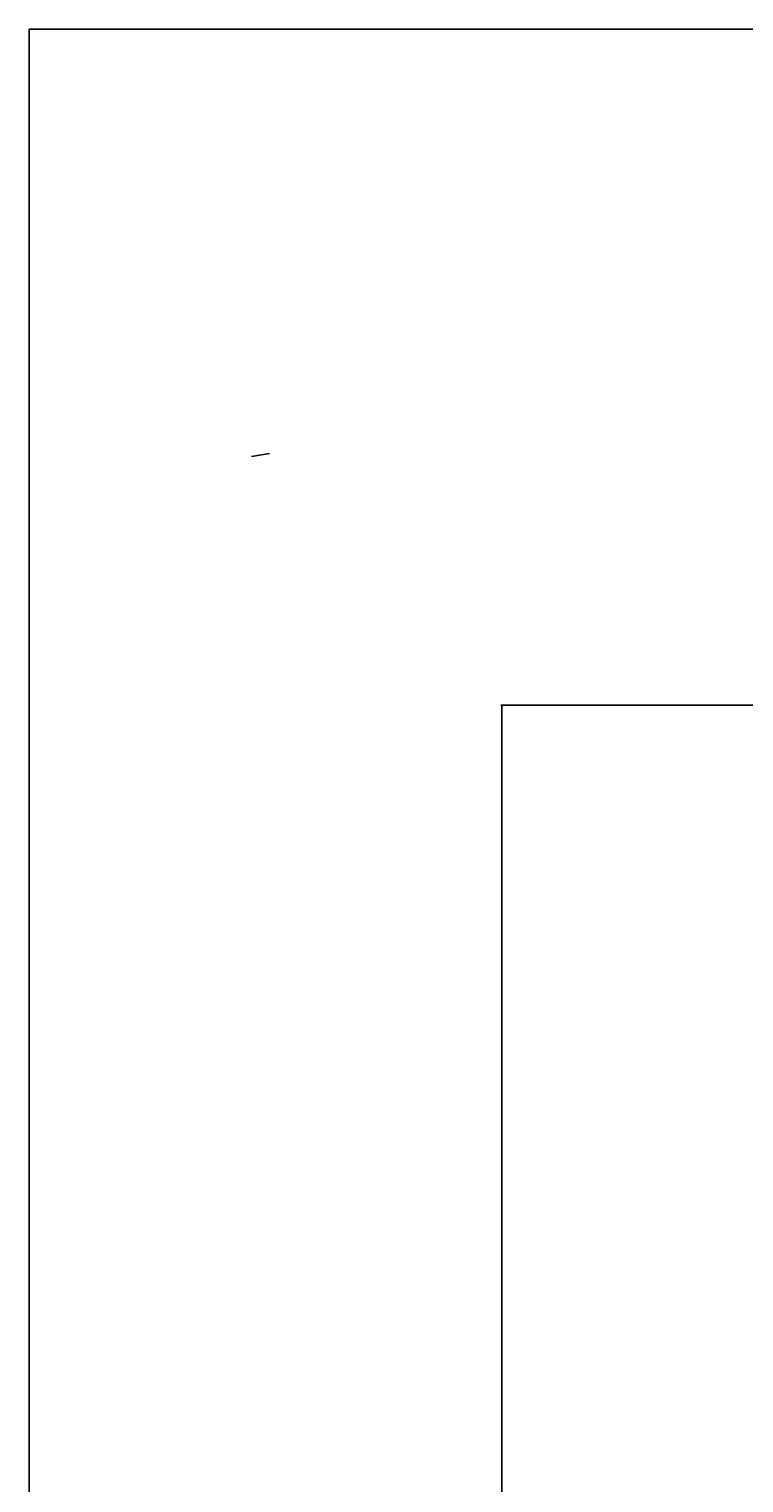
# Model space of a CAD drawing. Units: inches. Extents: x 2168 to 3056, y 1130 to 2629.
# Tile 22 of 42: x 2168 to 2327, y 2305 to 2629. Entities that reach past the tile are written whole.
import ezdxf

# ---------------------------------------------------------------- set-up
doc = ezdxf.new("R2010")
doc.units = ezdxf.units.IN
doc.layers.add('A-ANNO-DIMS', color=2, linetype='Continuous', lineweight=18)
doc.layers.add('A-ANNO-TTLB', color=7, linetype='Continuous', lineweight=25)
doc.styles.get("Standard").update_dxf_attribs({"font": 'arial.ttf'})
doc.dimstyles.get("Standard").update_dxf_attribs({"dimtxt": 0.18, "dimasz": 0.18, "dimexe": 0.18, "dimexo": 0.0625, "dimgap": 0.09, "dimtad": 0, "dimtih": 1, "dimtoh": 1, "dimdec": 4, "dimzin": 0, "dimdsep": 46, "dimtxsty": 'Standard', "dimcen": 0.09, "dimadec": 0, "dimazin": 0, "dimtfac": 1, "dimtdec": 4, "dimtofl": 0, "dimtmove": 0, "dimatfit": 3, "dimfxl": 1, "dimtolj": 1, "dimtzin": 0, "dimarcsym": 0})

# ---------------------------------------------------------------- blocks, each defined once
blk = doc.blocks.new('*D41')
at = {"layer": 'A-ANNO-DIMS', "color": 0, "lineweight": -2, "transparency": 16777216}
for p, q in [((2331.73, 2478.39), (2273.32, 2478.39)), ((2273.5, 2478.21), (2273.5, 1928.07)), ((2273.5, 1377.57), (2273.5, 1927.71)), ((2331.73, 1377.39), (2273.32, 1377.39))]:
    blk.add_line(p, q, dxfattribs=at)
at = {"layer": 'A-ANNO-DIMS', "color": 0, "transparency": 16777216}
for points in [[(2273.47, 2478.21), (2273.53, 2478.21), (2273.5, 2478.39)], [(2273.47, 1377.57), (2273.53, 1377.57), (2273.5, 1377.39)]]:
    blk.add_solid(points, dxfattribs=at)
at = {"layer": 'Defpoints', "color": 0, "transparency": 16777216}
for p in [(2273.5, 2478.39), (2331.8, 2478.39), (2331.8, 1377.39)]:
    blk.add_point(p, dxfattribs=at)
at = {"layer": 'A-ANNO-DIMS', "color": 0, "transparency": 16777216, "insert": (2273.5, 1927.89), "char_height": 0.18, "attachment_point": 5}
blk.add_mtext('\\A1;1101', dxfattribs=at)

msp = doc.modelspace()

# ---------------------------------------------------------------- linework, layer by layer
at = {"layer": 'A-ANNO-TTLB'}
msp.add_line((2217.71, 2533.89), (2221.74, 2534.56), dxfattribs=at)
msp.add_lwpolyline([(2168.16, 2629.19), (3055.63, 2629.19), (3055.63, 1130.19), (2168.16, 1130.19)], close=True, dxfattribs=at)

# ---------------------------------------------------------------- dimensions: what is measured, and where the dimension line sits
at = {"layer": 'A-ANNO-DIMS'}
dim = msp.add_linear_dim(base=(2273.5, 2478.39), p1=(2331.8, 1377.39), p2=(2331.8, 2478.39), angle=90, dimstyle='Standard', override={"dimdec": 0, "dimlfac": 1, "dimrnd": 0, "dimzin": 0, "dimdsep": 46, "dimlunit": 2}, dxfattribs=at)
dim.commit()
dim.dimension.update_dxf_attribs({"geometry": '*D41', "text_midpoint": (2273.5, 1927.89)})

doc.saveas('drawing.dxf')
